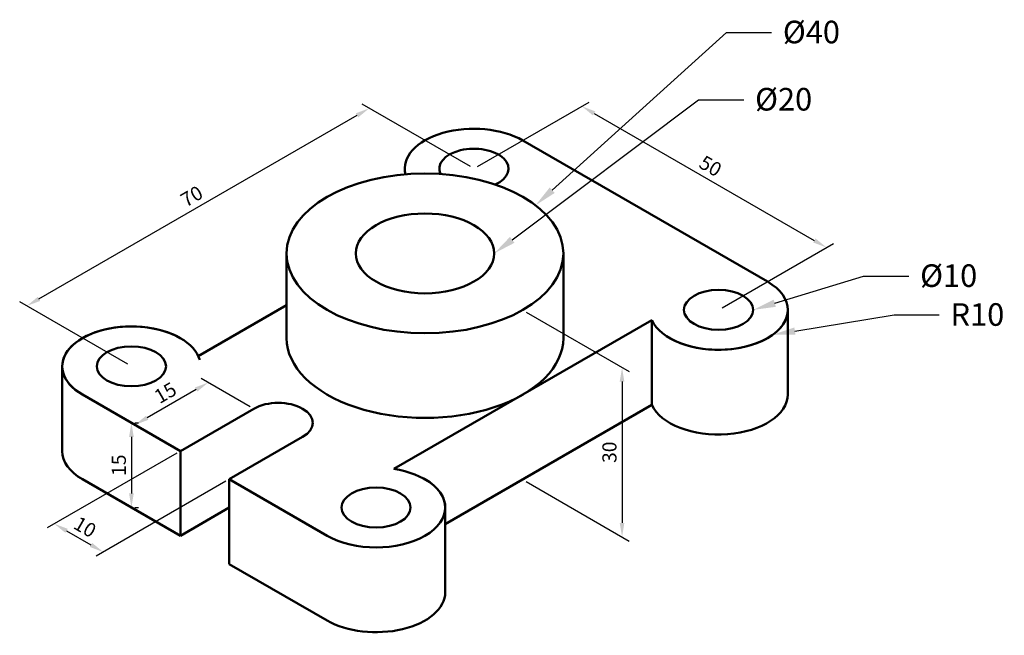
# Model space of a CAD drawing. Units: millimetres. Extents: x 2653 to 2827, y 1742 to 1851.
import ezdxf
from ezdxf import colors
from ezdxf.entities.mleader import LeaderData, LeaderLine
from ezdxf.math import Vec2, Vec3

# ---------------------------------------------------------------- set-up
doc = ezdxf.new("R2010")
doc.units = ezdxf.units.MM
doc.layers.add('M-DIMS', color=2, linetype='Continuous', lineweight=25)
doc.layers.add('M-OUTL', color=7, linetype='Continuous', lineweight=50)
doc.styles.get("Standard").update_dxf_attribs({"font": 'arial.ttf'})
doc.dimstyles.new('ISO-25', dxfattribs={"dimtxt": 2.5, "dimasz": 2.5, "dimexe": 1.25, "dimexo": 0.625, "dimtad": 1, "dimtxsty": 'Standard', "dimcen": 2.5, "dimadec": 0, "dimazin": 0, "dimtfac": 1, "dimtmove": 0, "dimatfit": 3, "dimfxl": 1, "dimarcsym": 0})

# ---------------------------------------------------------------- blocks, each defined once
blk = doc.blocks.new('*D1')
at = {"layer": 'Defpoints', "color": 0, "transparency": 16777216}
for p in [(2681.03, 1774.18), (2689.7, 1769.18), (2667.39, 1756.3)]:
    blk.add_point(p, dxfattribs=at)
at = {"layer": 'M-DIMS', "color": 0, "lineweight": -2, "transparency": 16777216}
for p, q in [((2680.41, 1773.82), (2657.48, 1760.58)), ((2689.07, 1768.82), (2666.14, 1755.58)), ((2660.89, 1760.05), (2665.22, 1757.55))]:
    blk.add_line(p, q, dxfattribs=at)
at = {"layer": 'M-DIMS', "color": 0, "transparency": 16777216}
for points in [[(2661.1, 1760.41), (2660.69, 1759.69), (2658.73, 1761.3)], [(2665.43, 1757.91), (2665.02, 1757.19), (2667.39, 1756.3)]]:
    blk.add_solid(points, dxfattribs=at)
at = {"layer": 'M-DIMS', "color": 0, "transparency": 16777216, "insert": (2664.01, 1760.45), "char_height": 2.5, "attachment_point": 5, "rotation": 330}
blk.add_mtext('10', dxfattribs=at)
blk = doc.blocks.new('*D2')
at = {"layer": 'Defpoints', "color": 0, "transparency": 16777216}
for p in [(2672.37, 1779.18), (2672.37, 1764.18), (2672.37, 1764.18)]:
    blk.add_point(p, dxfattribs=at)
at = {"layer": 'M-DIMS', "color": 0, "lineweight": -2, "transparency": 16777216}
for p, q in [((2673, 1779.18), (2673.62, 1779.18)), ((2672.37, 1776.68), (2672.37, 1766.68)), ((2673, 1764.18), (2673.62, 1764.18))]:
    blk.add_line(p, q, dxfattribs=at)
at = {"layer": 'M-DIMS', "color": 0, "transparency": 16777216}
for points in [[(2671.96, 1776.68), (2672.79, 1776.68), (2672.37, 1779.18)], [(2671.96, 1766.68), (2672.79, 1766.68), (2672.37, 1764.18)]]:
    blk.add_solid(points, dxfattribs=at)
at = {"layer": 'M-DIMS', "color": 0, "transparency": 16777216, "insert": (2670.47, 1771.68), "char_height": 2.5, "attachment_point": 5, "rotation": 90}
blk.add_mtext('15', dxfattribs=at)
blk = doc.blocks.new('*D3')
at = {"layer": 'Defpoints', "color": 0, "transparency": 16777216}
for p in [(2741.59, 1799.14), (2741.59, 1769.14), (2759.22, 1758.97)]:
    blk.add_point(p, dxfattribs=at)
at = {"layer": 'M-DIMS', "color": 0, "lineweight": -2, "transparency": 16777216}
for p, q in [((2742.22, 1798.78), (2760.47, 1788.25)), ((2759.22, 1786.47), (2759.22, 1761.47)), ((2742.22, 1768.78), (2760.47, 1758.25))]:
    blk.add_line(p, q, dxfattribs=at)
at = {"layer": 'M-DIMS', "color": 0, "transparency": 16777216}
for points in [[(2758.8, 1786.47), (2759.63, 1786.47), (2759.22, 1788.97)], [(2758.8, 1761.47), (2759.63, 1761.47), (2759.22, 1758.97)]]:
    blk.add_solid(points, dxfattribs=at)
at = {"layer": 'M-DIMS', "color": 0, "transparency": 16777216, "insert": (2757.31, 1773.97), "char_height": 2.5, "attachment_point": 5, "rotation": 90}
blk.add_mtext('30', dxfattribs=at)
blk = doc.blocks.new('*D4')
at = {"layer": 'Defpoints', "color": 0, "transparency": 16777216}
for p in [(2733, 1824.18), (2795.42, 1810.22), (2776.3, 1799.18)]:
    blk.add_point(p, dxfattribs=at)
at = {"layer": 'M-DIMS', "color": 0, "lineweight": -2, "transparency": 16777216}
for p, q in [((2733.62, 1824.54), (2753.37, 1835.94)), ((2754.28, 1833.97), (2793.25, 1811.47)), ((2776.92, 1799.54), (2796.67, 1810.94))]:
    blk.add_line(p, q, dxfattribs=at)
at = {"layer": 'M-DIMS', "color": 0, "transparency": 16777216}
for points in [[(2754.49, 1834.33), (2754.07, 1833.61), (2752.12, 1835.22)], [(2793.46, 1811.83), (2793.05, 1811.11), (2795.42, 1810.22)]]:
    blk.add_solid(points, dxfattribs=at)
at = {"layer": 'M-DIMS', "color": 0, "transparency": 16777216, "insert": (2774.72, 1824.37), "char_height": 2.5, "attachment_point": 5, "rotation": 330}
blk.add_mtext('50', dxfattribs=at)
blk = doc.blocks.new('*D5')
at = {"layer": 'Defpoints', "color": 0, "transparency": 16777216}
for p in [(2714.47, 1834.88), (2733, 1824.18), (2672.37, 1789.18)]:
    blk.add_point(p, dxfattribs=at)
at = {"layer": 'M-DIMS', "color": 0, "lineweight": -2, "transparency": 16777216}
for p, q in [((2732.37, 1824.54), (2713.22, 1835.6)), ((2656.01, 1801.13), (2712.31, 1833.63)), ((2671.75, 1789.54), (2652.6, 1800.6))]:
    blk.add_line(p, q, dxfattribs=at)
at = {"layer": 'M-DIMS', "color": 0, "transparency": 16777216}
for points in [[(2712.1, 1833.99), (2712.51, 1833.26), (2714.47, 1834.88)], [(2655.81, 1801.49), (2656.22, 1800.76), (2653.85, 1799.88)]]:
    blk.add_solid(points, dxfattribs=at)
at = {"layer": 'M-DIMS', "color": 0, "transparency": 16777216, "insert": (2683.21, 1819.02), "char_height": 2.5, "attachment_point": 5, "rotation": 30}
blk.add_mtext('70', dxfattribs=at)
blk = doc.blocks.new('*D6')
at = {"layer": 'Defpoints', "color": 0, "transparency": 16777216}
for p in [(2694.03, 1781.68), (2673, 1778.82), (2681.03, 1774.18)]:
    blk.add_point(p, dxfattribs=at)
at = {"layer": 'M-DIMS', "color": 0, "lineweight": -2, "transparency": 16777216}
for p, q in [((2693.4, 1782.04), (2684.74, 1787.04)), ((2683.82, 1785.07), (2675.16, 1780.07)), ((2680.41, 1774.54), (2671.75, 1779.54))]:
    blk.add_line(p, q, dxfattribs=at)
at = {"layer": 'M-DIMS', "color": 0, "transparency": 16777216}
for points in [[(2683.62, 1785.43), (2684.03, 1784.71), (2685.99, 1786.32)], [(2674.96, 1780.43), (2675.37, 1779.71), (2673, 1778.82)]]:
    blk.add_solid(points, dxfattribs=at)
at = {"layer": 'M-DIMS', "color": 0, "transparency": 16777216, "insert": (2678.54, 1784.22), "char_height": 2.5, "attachment_point": 5, "rotation": 30}
blk.add_mtext('15', dxfattribs=at)

msp = doc.modelspace()

# ---------------------------------------------------------------- linework, layer by layer
at = {"layer": 'M-OUTL'}
for p, q in [((2741.657, 1829.18), (2784.958, 1804.18)), ((2699.841, 1809.18), (2699.841, 1794.18)), ((2748.831, 1809.18), (2748.831, 1794.18)), ((2684.205, 1791.01), (2699.841, 1800.038)), ((2788.545, 1799.18), (2788.545, 1784.18)), ((2764.467, 1797.35), (2718.846, 1771.01)), ((2764.467, 1782.35), (2764.467, 1797.35)), ((2660.127, 1789.18), (2660.127, 1774.18)), ((2681.035, 1774.18), (2663.714, 1784.18)), ((2694.025, 1781.68), (2681.035, 1774.18)), ((2727.923, 1761.251), (2764.467, 1782.35)), ((2689.695, 1769.18), (2702.685, 1776.68)), ((2681.035, 1774.18), (2681.035, 1759.18)), ((2681.035, 1759.18), (2663.714, 1769.18)), ((2707.016, 1759.18), (2689.695, 1769.18)), ((2689.695, 1769.18), (2689.695, 1754.18)), ((2689.695, 1764.18), (2681.035, 1759.18)), ((2727.923, 1749.18), (2727.923, 1764.18)), ((2707.016, 1744.18), (2689.695, 1754.18))]:
    msp.add_line(p, q, dxfattribs=at)
for centre, major_axis, start_param, end_param in [((2732.996, 1824.18), (-12.247, 0), 3.9269908, 6.4250824), ((2732.996, 1824.18), (-12.247, 0), 3.9269908, 6.4250824), ((2732.996, 1824.18), (-6.124, 0), 2.2266423, 6.5546345), ((2776.298, 1799.18), (-12.247, 0), 0.7853982, 3.9269908), ((2776.298, 1799.18), (-12.247, 0), 0.2617994, 3.1415927), ((2672.375, 1789.18), (-12.247, 0), 3.3034464, 7.0685835), ((2672.375, 1789.18), (-12.247, 0), 3.9269908, 7.0685835), ((2724.336, 1794.18), (-24.495, 0), 6.2831853, 9.424778), ((2698.355, 1779.18), (-6.124, 0), 2.3561945, 5.4977871), ((2776.298, 1784.18), (-12.247, 0), 0.2617994, 3.1415927), ((2672.375, 1774.18), (-12.247, 0), 6.2831853, 7.0685835), ((2715.676, 1764.18), (-12.247, 0), 3.1415927, 4.4505896), ((2715.676, 1764.18), (-12.247, 0), 0.7853982, 3.9269908), ((2715.676, 1749.18), (-12.247, 0), 0.7853982, 3.1415927), ((2715.676, 1749.18), (-12.247, 0), 0.7853982, 3.1415927)]:
    msp.add_ellipse(centre, major_axis=major_axis, ratio=0.5773503, start_param=start_param, end_param=end_param, dxfattribs=at)
for centre, major_axis in [((2724.336, 1809.18), (-24.495, 0)), ((2724.336, 1809.18), (-12.247, 0)), ((2776.298, 1799.18), (-6.124, 0)), ((2672.375, 1789.18), (-6.124, 0)), ((2715.676, 1764.18), (-6.124, 0))]:
    msp.add_ellipse(centre, major_axis=major_axis, ratio=0.5773503, dxfattribs=at)

# ---------------------------------------------------------------- dimensions: what is measured, and where the dimension line sits
at = {"layer": 'M-DIMS'}
for p1, p2, distance, picture, middle in [((2672.375, 1789.18), (2732.996, 1824.18), 18.525, '*D5', (2683.21, 1819.022)), ((2732.996, 1824.18), (2776.298, 1799.18), 19.121, '*D4', (2774.719, 1824.367)), ((2741.595, 1799.145), (2741.595, 1769.145), 17.621, '*D3', (2757.314, 1773.971)), ((2694.025, 1781.68), (2681.035, 1774.18), -8.035, '*D6', (2678.544, 1784.216)), ((2672.375, 1779.18), (2672.375, 1764.18), 0, '*D2', (2670.473, 1771.68)), ((2681.035, 1774.18), (2689.695, 1769.18), -22.306, '*D1', (2664.01, 1760.449))]:
    dim = msp.add_aligned_dim(p1=p1, p2=p2, distance=distance, dimstyle='ISO-25', override={"dimclrd": 0, "dimclre": 0, "dimclrt": 0}, dxfattribs=at)
    dim.commit()
    dim.dimension.update_dxf_attribs({"geometry": picture, "text_midpoint": middle})

# ---------------------------------------------------------------- leaders
ml = msp.add_multileader_mtext('Standard', dxfattribs=at)
ml.set_content('%%C40', color=256)
ml.set_leader_properties()
ml.build(insert=Vec2(0, 0))
ctx = ml.context
ctx.base_point, ctx.plane_origin = Vec3(2785.683, 1848.3), Vec3(2743.898, 1817.691)
notes = []
notes.append((ctx, [(0, (1, 1, 0), (2777.683, 1848.3), (1, 0), 8, [(0, [(2743.898, 1817.691)], 0, [])])]))
ctx.mtext.insert, ctx.mtext.flow_direction = Vec3(2787.683, 1850.381), 5
ml = msp.add_multileader_mtext('Standard', dxfattribs=at)
ml.set_content('%%C20', color=256)
ml.set_leader_properties()
ml.build(insert=Vec2(0, 0))
ctx = ml.context
ctx.base_point, ctx.plane_origin = Vec3(2780.763, 1836.398), Vec3(2736.584, 1809.18)
notes.append((ctx, [(0, (1, 1, 0), (2772.763, 1836.398), (1, 0), 8, [(0, [(2736.584, 1809.18)], 0, [])])]))
ctx.mtext.insert, ctx.mtext.flow_direction = Vec3(2782.763, 1838.478), 5
ml = msp.add_multileader_mtext('Standard', dxfattribs=at)
ml.set_content('%%C10', color=256)
ml.set_leader_properties()
ml.build(insert=Vec2(0, 0))
ctx = ml.context
ctx.base_point, ctx.plane_origin = Vec3(2809.979, 1805.16), Vec3(2782.421, 1799.18)
notes.append((ctx, [(0, (1, 1, 0), (2801.979, 1805.16), (1, 0), 8, [(0, [(2782.421, 1799.18)], 0, [])])]))
ctx.mtext.insert, ctx.mtext.flow_direction = Vec3(2811.979, 1807.241), 5
ml = msp.add_multileader_mtext('Standard', dxfattribs=at)
ml.set_content('R10', color=256)
ml.set_leader_properties()
ml.build(insert=Vec2(0, 0))
ctx = ml.context
ctx.base_point, ctx.plane_origin = Vec3(2815.355, 1798.325), Vec3(2785.864, 1794.765)
notes.append((ctx, [(0, (1, 1, 0), (2807.355, 1798.325), (1, 0), 8, [(0, [(2785.864, 1794.765)], 0, [])])]))
ctx.mtext.insert, ctx.mtext.flow_direction = Vec3(2817.355, 1800.359), 5
for ctx, leaders in notes:
    for number, flags, end, landing, length, lines in leaders:
        leader = LeaderData()
        leader.index, (leader.has_last_leader_line, leader.has_dogleg_vector, leader.attachment_direction) = number, flags
        leader.last_leader_point, leader.dogleg_vector, leader.dogleg_length = Vec3(end), Vec3(landing), length
        for number, points, colour, breaks in lines:
            line = LeaderLine()
            line.index, line.vertices, line.color, line.breaks = number, Vec3.list(points), colors.encode_raw_color(colour), breaks
            leader.lines.append(line)
        ctx.leaders.append(leader)

doc.saveas('drawing.dxf')
